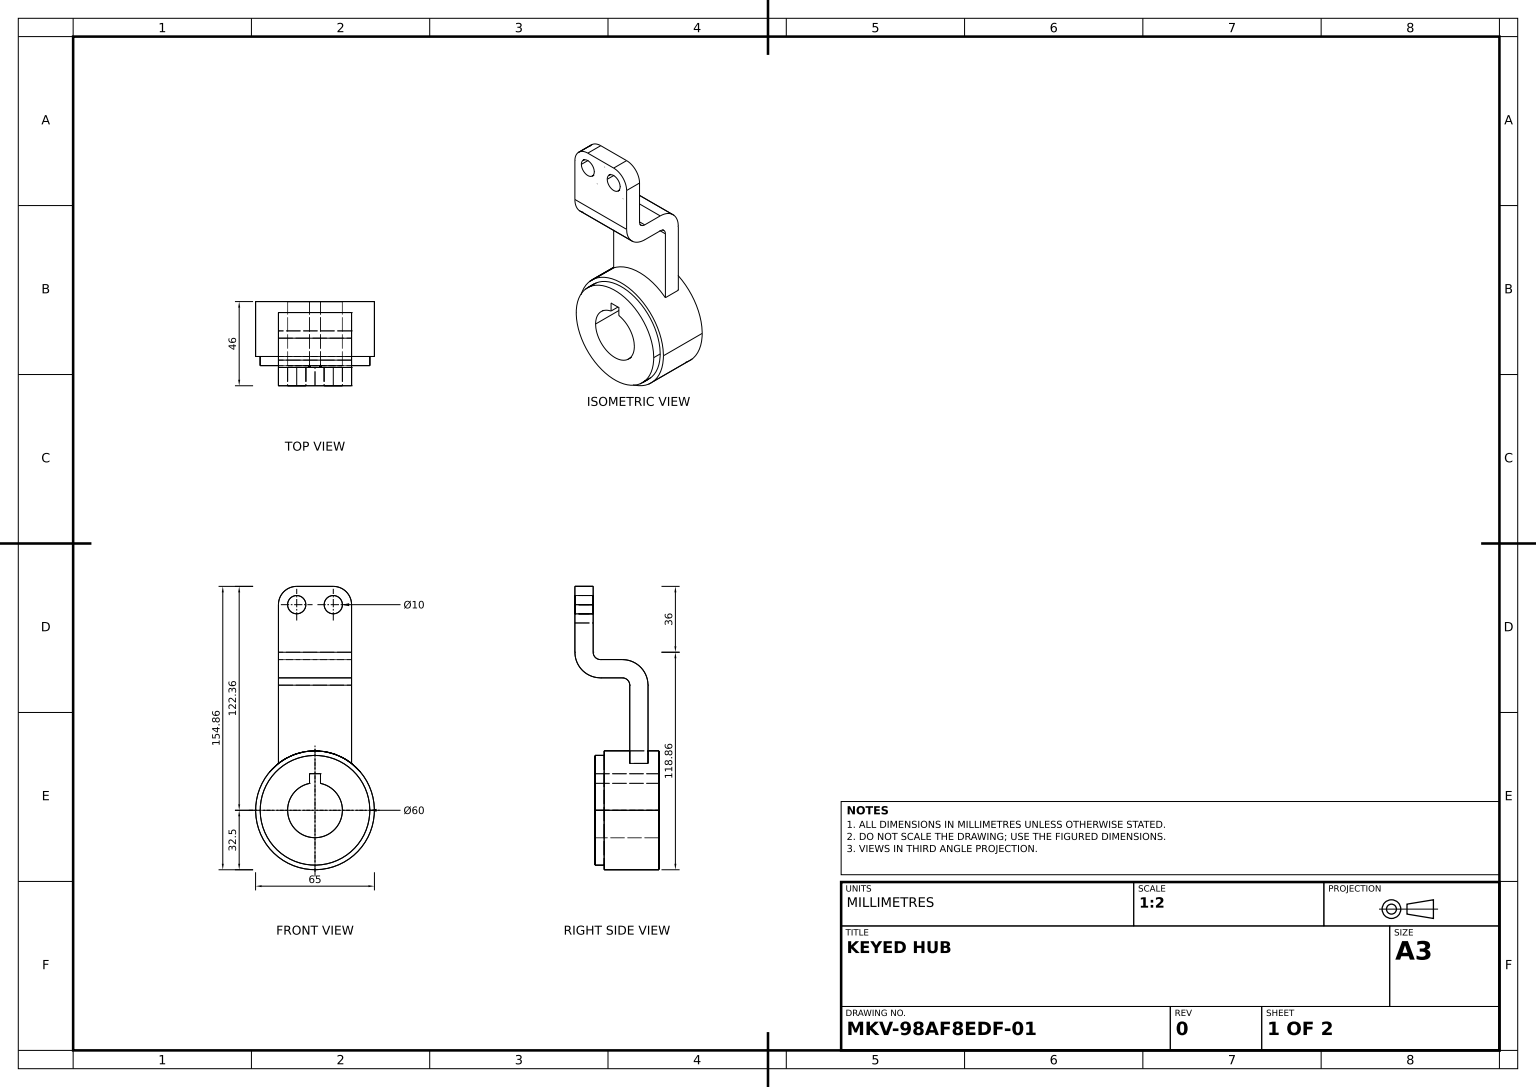
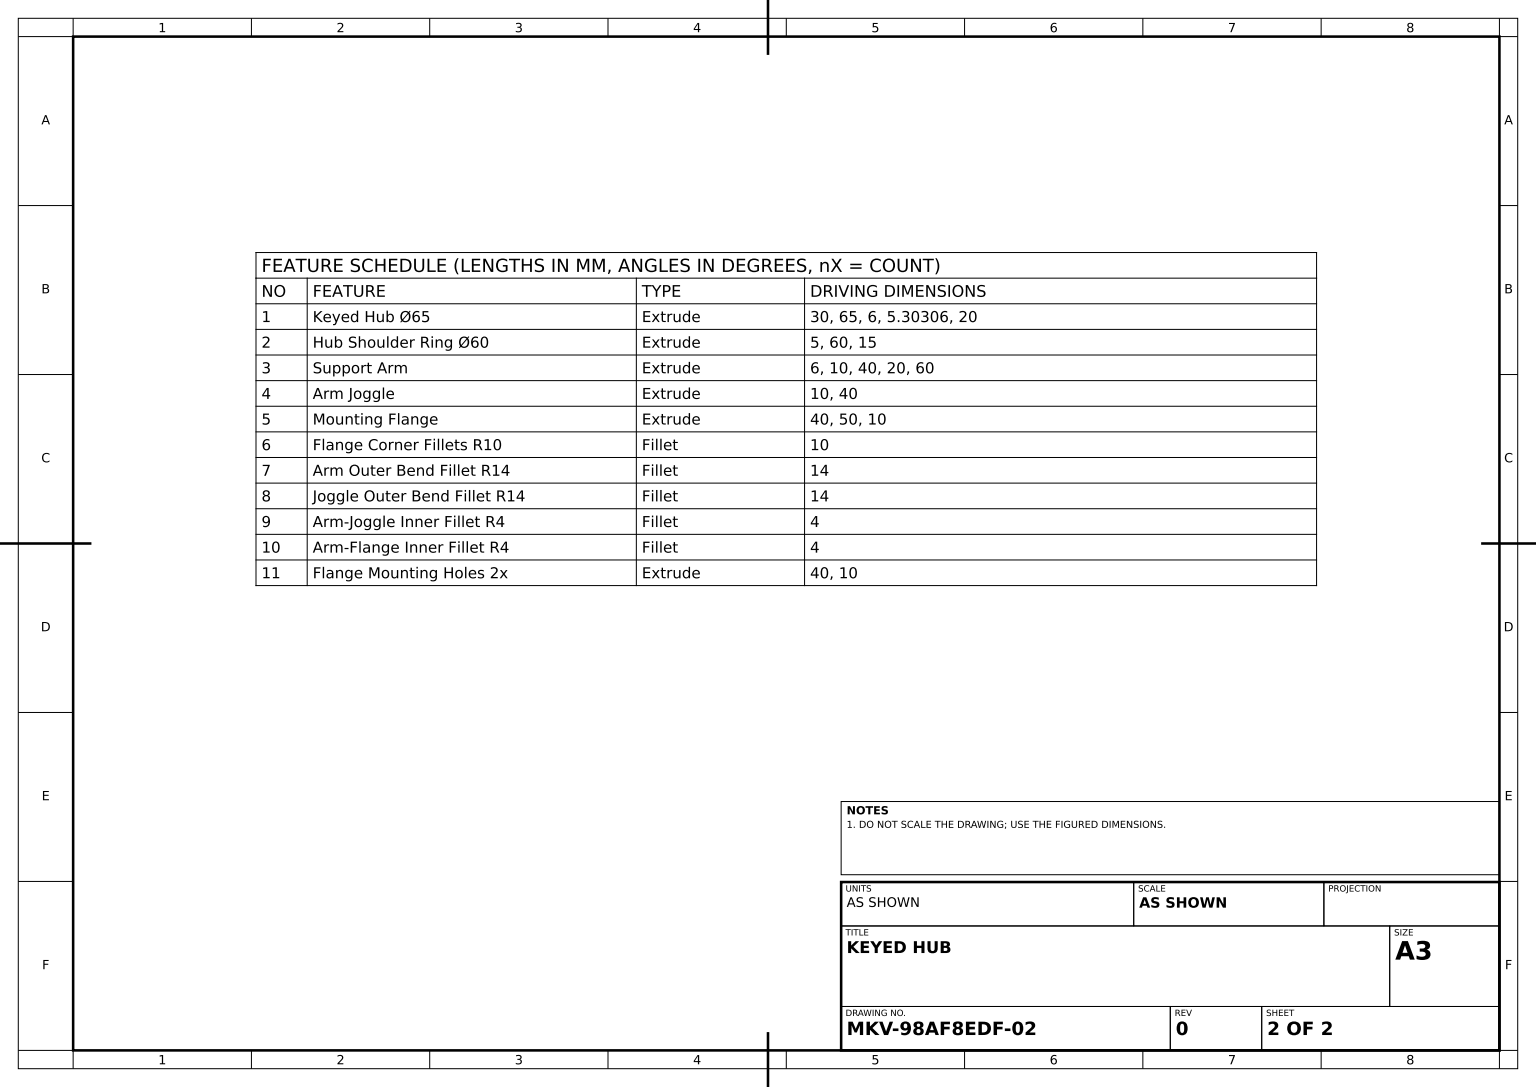
SolidWorks part; units mm, degrees
material "Plain Carbon Steel"
ref_plane "Front Plane" through (0, 0, 0) normal (0, 0, 1) x (1, 0, 0)
ref_plane "Top Plane" through (0, 0, 0) normal (0, 1, 0) x (1, 0, 0)
ref_plane "Right Plane" through (0, 0, 0) normal (1, 0, 0) x (0, 0, -1)
sketch "Keyed Hub Profile" plane through (0, 0, 0) normal (0, 0, 1) x (1, 0, 0)
  line L0 (-3, 20) -> (3, 20)
  line L1 (3, 14.6969) -> (3, 20)
  line L2 (-3, 14.6969) -> (-3, 20)
  circle A0 centre (0, 0) radius 32.5
  arc A1 (-3, 14.6969) -> (3, 14.6969) centre (0, 0) ccw
  point P4 (3, 0)
  point P5 (0, 20)
  point P7 (-3, 0)
  dimension "D1" = 65
  dimension "D2" = 30
  dimension "D3" = 6
  dimension "D4" = 5.3031
  dimension "D5" = 20
extrude "Keyed Hub Ø65" add sketch "Keyed Hub Profile" along normal blind 30
sketch "Hub Shoulder Profile" plane through (0, 0, 30) normal (0, 0, 1) x (1, 0, 0)
  line L0 (-3, 14.6969) -> (-3, 20)
  line L1 (-3, 20) -> (3, 20)
  line L2 (3, 20) -> (3, 14.6969)
  circle A0 centre (0, 0) radius 30
  arc A1 (-3, 14.6969) -> (3, 14.6969) centre (0, 0) ccw
  dimension "D1" = 60
  dimension "D2" = 15
extrude "Hub Shoulder Ring Ø60" add sketch "Hub Shoulder Profile" along normal blind 5
ref_plane "Arm Sketch Plane" through (0, 0, 6) normal (0, 0, 1) x (1, 0, 0)
sketch "Support Arm Profile" plane through (0, 0, 6) normal (0, 0, 1) x (1, 0, 0)
  line L0 (-20, 22.3607) -> (20, 22.3607)
  line L1 (-20, 22.3607) -> (-20, 82.3607)
  line L2 (-20, 82.3607) -> (20, 82.3607)
  line L3 (20, 82.3607) -> (20, 22.3607)
  circle A0 centre (0, 0) radius 30 construction
  point P5 (0, 22.3607)
  dimension "D1" = 40
  dimension "D2" = 20
  dimension "D3" = 60
extrude "Support Arm" add sketch "Support Arm Profile" along normal blind 10
sketch "Arm Joggle Profile" plane through (0, 82.3607, 0) normal (0, 1, 0) x (1, 0, 0)
  line L1 (-20, -6) -> (20, -6)
  line L2 (-20, -6) -> (-20, -46)
  line L3 (-20, -46) -> (20, -46)
  line L4 (20, -6) -> (20, -46)
  dimension "D1" = 40
extrude "Arm Joggle" add sketch "Arm Joggle Profile" against normal blind 10
sketch "Mounting Flange Profile" plane through (20, 0, 0) normal (1, 0, 0) x (0, 0, -1)
  line L1 (-46, 72.3607) -> (-36, 72.3607)
  line L2 (-46, 72.3607) -> (-46, 122.3607)
  line L3 (-46, 122.3607) -> (-36, 122.3607)
  line L4 (-36, 72.3607) -> (-36, 122.3607)
  dimension "D1" = 50
  dimension "D2" = 10
extrude "Mounting Flange" add sketch "Mounting Flange Profile" against normal blind 40
fillet "Flange Corner Fillets R10" radius 10 2 edges at (20, 122.3607, 41) (-20, 122.3607, 41)
fillet "Arm Outer Bend Fillet R14" radius 14 1 edges at (0, 82.3607, 6)
fillet "Joggle Outer Bend Fillet R14" radius 14 1 edges at (0, 72.3607, 46)
fillet "Arm-Joggle Inner Fillet R4" radius 4 1 edges at (0, 72.3607, 16)
fillet "Arm-Flange Inner Fillet R4" radius 4 1 edges at (0, 82.3607, 36)
sketch "Flange Mounting Holes Profile" plane through (0, 0, 46) normal (0, 0, 1) x (1, 0, 0)
  circle A0 centre (-10, 112.3607) radius 5
  circle A1 centre (10, 112.3607) radius 5
  dimension "D1" = 10
  dimension "D2" = 10
extrude "Flange Mounting Holes 2x" cut sketch "Flange Mounting Holes Profile" against normal blind 40
